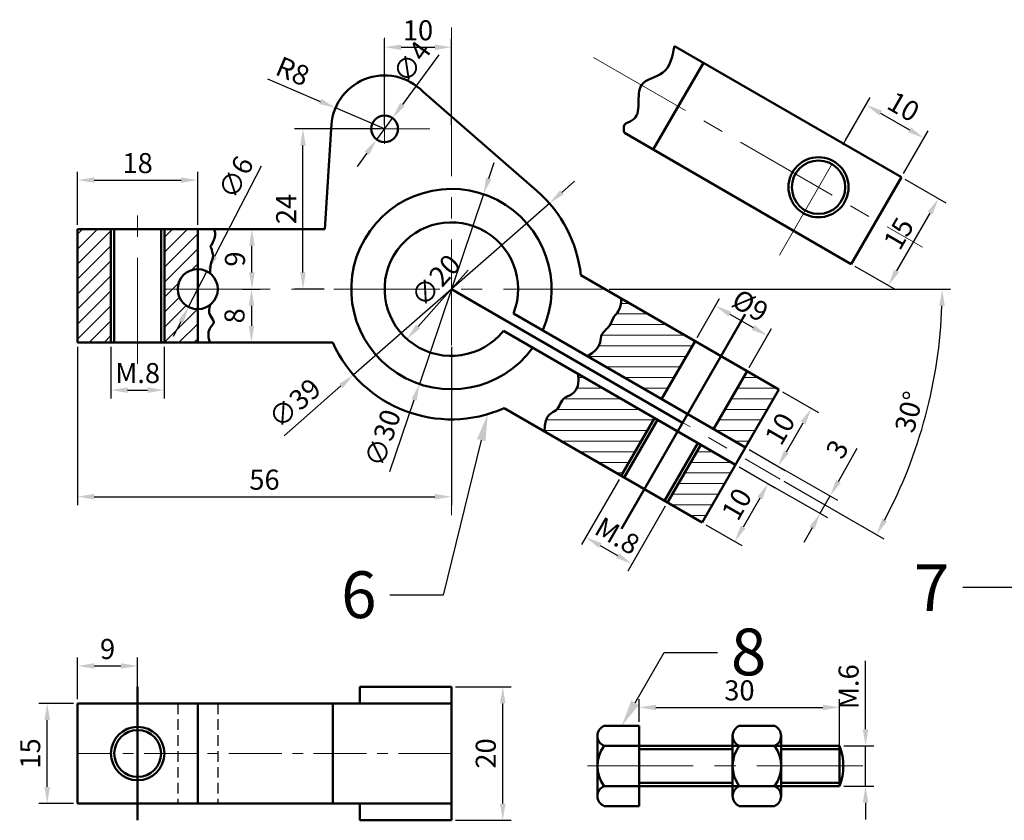
# Model space of a CAD drawing. Units: millimetres. Extents: x 77 to 718, y -35 to 313.
# Tile 5 of 7: x 386 to 533, y 99 to 219. Entities that reach past the tile are written whole.
import ezdxf
from ezdxf import colors
from ezdxf.entities.mleader import LeaderData, LeaderLine
from ezdxf.math import Vec2, Vec3

# ---------------------------------------------------------------- set-up
doc = ezdxf.new("R2010")
doc.units = ezdxf.units.MM
doc.header["$LTSCALE"] = 0.5
doc.linetypes.add('CENTER', pattern=[50.8, 31.75, -6.35, 6.35, -6.35])
doc.linetypes.add('HIDDEN', pattern=[9.525, 6.35, -3.175])
for name, color, linetype, lineweight in [('M-CNTR', 1, 'CENTER', 18), ('M-DIMS', 2, 'Continuous', 25), ('M-HATC', 8, 'Continuous', 18), ('M-HIDN', 8, 'HIDDEN', 25), ('M-OUTL', 7, 'Continuous', 50), ('M-TEXT', 3, 'Continuous', 25)]:
    doc.layers.add(name, color=color, linetype=linetype, lineweight=lineweight)
doc.styles.get("Standard").update_dxf_attribs({"font": 'arial.ttf'})
doc.dimstyles.new('ISO-25', dxfattribs={"dimtxt": 3, "dimasz": 2.5, "dimexe": 1.25, "dimexo": 0.625, "dimtad": 1, "dimtxsty": 'Standard', "dimcen": 2.5, "dimadec": 0, "dimazin": 0, "dimtfac": 1, "dimtmove": 0, "dimatfit": 3, "dimfxl": 1, "dimarcsym": 0})

# ---------------------------------------------------------------- blocks, each defined once
blk = doc.blocks.new('*D67')
at = {"layer": 'Defpoints', "color": 0, "transparency": 16777216}
for p in [(412.28, 195.29), (394.28, 187.97), (412.28, 187.97)]:
    blk.add_point(p, dxfattribs=at)
at = {"layer": 'M-DIMS', "color": 0, "lineweight": -2, "transparency": 16777216}
for p, q in [((394.28, 188.59), (394.28, 196.54)), ((412.28, 188.59), (412.28, 196.54)), ((396.78, 195.29), (409.78, 195.29))]:
    blk.add_line(p, q, dxfattribs=at)
at = {"layer": 'M-DIMS', "color": 0, "transparency": 16777216}
for points in [[(396.78, 195.71), (396.78, 194.88), (394.28, 195.29)], [(409.78, 195.71), (409.78, 194.88), (412.28, 195.29)]]:
    blk.add_solid(points, dxfattribs=at)
at = {"layer": 'M-DIMS', "color": 0, "transparency": 16777216, "insert": (403.28, 197.45), "char_height": 3, "attachment_point": 5}
blk.add_mtext('18', dxfattribs=at)
blk = doc.blocks.new('*D68')
at = {"layer": 'Defpoints', "color": 0, "transparency": 16777216}
for p in [(428.05, 202.97), (440.28, 202.97), (431.83, 178.97)]:
    blk.add_point(p, dxfattribs=at)
at = {"layer": 'M-DIMS', "color": 0, "lineweight": -2, "transparency": 16777216}
for p, q in [((439.66, 202.97), (426.8, 202.97)), ((428.05, 181.47), (428.05, 200.47)), ((431.21, 178.97), (426.8, 178.97))]:
    blk.add_line(p, q, dxfattribs=at)
at = {"layer": 'M-DIMS', "color": 0, "transparency": 16777216}
for points in [[(427.64, 200.47), (428.47, 200.47), (428.05, 202.97)], [(427.64, 181.47), (428.47, 181.47), (428.05, 178.97)]]:
    blk.add_solid(points, dxfattribs=at)
at = {"layer": 'M-DIMS', "color": 0, "transparency": 16777216, "insert": (425.92, 190.97), "char_height": 3, "attachment_point": 5, "rotation": 90}
blk.add_mtext('24', dxfattribs=at)
blk = doc.blocks.new('*D69')
at = {"layer": 'Defpoints', "color": 0, "transparency": 16777216}
for p in [(450.28, 215.19), (440.28, 202.97), (450.28, 202.97)]:
    blk.add_point(p, dxfattribs=at)
at = {"layer": 'M-DIMS', "color": 0, "lineweight": -2, "transparency": 16777216}
for p, q in [((440.28, 203.59), (440.28, 216.44)), ((450.28, 203.59), (450.28, 216.44)), ((442.78, 215.19), (447.78, 215.19))]:
    blk.add_line(p, q, dxfattribs=at)
at = {"layer": 'M-DIMS', "color": 0, "transparency": 16777216}
for points in [[(442.78, 215.6), (442.78, 214.77), (440.28, 215.19)], [(447.78, 215.6), (447.78, 214.77), (450.28, 215.19)]]:
    blk.add_solid(points, dxfattribs=at)
at = {"layer": 'M-DIMS', "color": 0, "transparency": 16777216, "insert": (445.28, 217.34), "char_height": 3, "attachment_point": 5}
blk.add_mtext('10', dxfattribs=at)
blk = doc.blocks.new('*D70')
at = {"layer": 'Defpoints', "color": 0, "transparency": 16777216}
for p in [(399.28, 170.97), (407.28, 170.97), (407.28, 163.85)]:
    blk.add_point(p, dxfattribs=at)
at = {"layer": 'M-DIMS', "color": 0, "lineweight": -2, "transparency": 16777216}
for p, q in [((399.28, 170.34), (399.28, 162.6)), ((407.28, 170.34), (407.28, 162.6)), ((401.78, 163.85), (404.78, 163.85))]:
    blk.add_line(p, q, dxfattribs=at)
at = {"layer": 'M-DIMS', "color": 0, "transparency": 16777216}
for points in [[(401.78, 164.27), (401.78, 163.43), (399.28, 163.85)], [(404.78, 164.27), (404.78, 163.43), (407.28, 163.85)]]:
    blk.add_solid(points, dxfattribs=at)
at = {"layer": 'M-DIMS', "color": 0, "transparency": 16777216, "insert": (403.28, 166.01), "char_height": 3, "attachment_point": 5}
blk.add_mtext('M.8', dxfattribs=at)
blk = doc.blocks.new('*D71')
at = {"layer": 'Defpoints', "color": 0, "transparency": 16777216}
for p in [(418.39, 187.97), (420.41, 187.97), (418.39, 178.97)]:
    blk.add_point(p, dxfattribs=at)
at = {"layer": 'M-DIMS', "color": 0, "lineweight": -2, "transparency": 16777216}
for p, q in [((419.01, 187.97), (421.66, 187.97)), ((420.41, 181.47), (420.41, 185.47)), ((419.01, 178.97), (421.66, 178.97))]:
    blk.add_line(p, q, dxfattribs=at)
at = {"layer": 'M-DIMS', "color": 0, "transparency": 16777216}
for points in [[(419.99, 185.47), (420.82, 185.47), (420.41, 187.97)], [(419.99, 181.47), (420.82, 181.47), (420.41, 178.97)]]:
    blk.add_solid(points, dxfattribs=at)
at = {"layer": 'M-DIMS', "color": 0, "transparency": 16777216, "insert": (418.25, 183.47), "char_height": 3, "attachment_point": 5, "rotation": 90}
blk.add_mtext('9', dxfattribs=at)
blk = doc.blocks.new('*D72')
at = {"layer": 'Defpoints', "color": 0, "transparency": 16777216}
for p in [(420.33, 178.97), (420.33, 170.97), (420.33, 170.97)]:
    blk.add_point(p, dxfattribs=at)
at = {"layer": 'M-DIMS', "color": 0, "lineweight": -2, "transparency": 16777216}
for p, q in [((420.96, 178.97), (421.58, 178.97)), ((420.33, 176.47), (420.33, 173.47)), ((420.96, 170.97), (421.58, 170.97))]:
    blk.add_line(p, q, dxfattribs=at)
at = {"layer": 'M-DIMS', "color": 0, "transparency": 16777216}
for points in [[(419.92, 176.47), (420.75, 176.47), (420.33, 178.97)], [(419.92, 173.47), (420.75, 173.47), (420.33, 170.97)]]:
    blk.add_solid(points, dxfattribs=at)
at = {"layer": 'M-DIMS', "color": 0, "transparency": 16777216, "insert": (418.18, 174.97), "char_height": 3, "attachment_point": 5, "rotation": 90}
blk.add_mtext('8', dxfattribs=at)
blk = doc.blocks.new('*D73')
at = {"layer": 'Defpoints', "color": 0, "transparency": 16777216}
for p in [(499.34, 163.93), (504.21, 161.11), (494.34, 155.27)]:
    blk.add_point(p, dxfattribs=at)
at = {"layer": 'M-DIMS', "color": 0, "lineweight": -2, "transparency": 16777216}
for p, q in [((499.88, 163.61), (505.29, 160.49)), ((500.46, 154.62), (502.96, 158.95)), ((494.88, 154.95), (500.29, 151.83))]:
    blk.add_line(p, q, dxfattribs=at)
at = {"layer": 'M-DIMS', "color": 0, "transparency": 16777216}
for points in [[(502.6, 159.16), (503.32, 158.74), (504.21, 161.11)], [(500.1, 154.83), (500.82, 154.41), (499.21, 152.45)]]:
    blk.add_solid(points, dxfattribs=at)
at = {"layer": 'M-DIMS', "color": 0, "transparency": 16777216, "insert": (499.84, 157.86), "char_height": 3, "attachment_point": 5, "rotation": 60}
blk.add_mtext('10', dxfattribs=at)
blk = doc.blocks.new('*D74')
at = {"layer": 'Defpoints', "color": 0, "transparency": 16777216}
for p in [(492.84, 152.67), (487.84, 144.01), (492.73, 141.18)]:
    blk.add_point(p, dxfattribs=at)
at = {"layer": 'M-DIMS', "color": 0, "lineweight": -2, "transparency": 16777216}
for p, q in [((493.38, 152.36), (498.81, 149.22)), ((496.48, 147.68), (493.98, 143.35)), ((488.38, 143.7), (493.81, 140.56))]:
    blk.add_line(p, q, dxfattribs=at)
at = {"layer": 'M-DIMS', "color": 0, "transparency": 16777216}
for points in [[(496.12, 147.89), (496.84, 147.47), (497.73, 149.84)], [(493.62, 143.56), (494.34, 143.14), (492.73, 141.18)]]:
    blk.add_solid(points, dxfattribs=at)
at = {"layer": 'M-DIMS', "color": 0, "transparency": 16777216, "insert": (493.36, 146.59), "char_height": 3, "attachment_point": 5, "rotation": 60}
blk.add_mtext('10', dxfattribs=at)
blk = doc.blocks.new('*D75')
at = {"layer": 'Defpoints', "color": 0, "transparency": 16777216}
for p in [(499.21, 152.45), (497.73, 149.84), (507.03, 148.01)]:
    blk.add_point(p, dxfattribs=at)
at = {"layer": 'M-DIMS', "color": 0, "lineweight": -2, "transparency": 16777216}
for p, q in [((508.26, 150.18), (511.09, 155.15)), ((499.75, 152.14), (508.11, 147.39)), ((498.27, 149.54), (506.63, 144.78)), ((505.54, 145.4), (507.03, 148.01)), ((504.31, 143.23), (503.07, 141.05))]:
    blk.add_line(p, q, dxfattribs=at)
at = {"layer": 'M-DIMS', "color": 0, "transparency": 16777216}
for points in [[(507.9, 150.39), (508.62, 149.97), (507.03, 148.01)], [(503.94, 143.43), (504.67, 143.02), (505.54, 145.4)]]:
    blk.add_solid(points, dxfattribs=at)
at = {"layer": 'M-DIMS', "color": 0, "transparency": 16777216, "insert": (508.42, 154.82), "char_height": 3, "attachment_point": 5, "rotation": 60.3651}
blk.add_mtext('3', dxfattribs=at)
blk = doc.blocks.new('*D76')
at = {"layer": 'Defpoints', "color": 0, "transparency": 16777216}
for p in [(486.78, 171.18), (497.63, 171.98), (494.57, 166.68)]:
    blk.add_point(p, dxfattribs=at)
at = {"layer": 'M-DIMS', "color": 0, "lineweight": -2, "transparency": 16777216}
for p, q in [((487.09, 171.72), (490.46, 177.56)), ((492, 175.23), (495.47, 173.23)), ((494.88, 167.22), (498.26, 173.06))]:
    blk.add_line(p, q, dxfattribs=at)
at = {"layer": 'M-DIMS', "color": 0, "transparency": 16777216}
for points in [[(492.21, 175.59), (491.8, 174.87), (489.84, 176.48)], [(495.68, 173.59), (495.26, 172.87), (497.63, 171.98)]]:
    blk.add_solid(points, dxfattribs=at)
at = {"layer": 'M-DIMS', "color": 0, "transparency": 16777216, "insert": (494.86, 176.17), "char_height": 3, "attachment_point": 5, "rotation": 330}
blk.add_mtext('%%C9', dxfattribs=at)
blk = doc.blocks.new('*D77')
at = {"layer": 'Defpoints', "color": 0, "transparency": 16777216}
for p in [(517.69, 195.72), (523.24, 192.51), (510.19, 182.73)]:
    blk.add_point(p, dxfattribs=at)
at = {"layer": 'M-DIMS', "color": 0, "lineweight": -2, "transparency": 16777216}
for p, q in [((518.23, 195.41), (524.33, 191.89)), ((516.99, 181.69), (521.99, 190.35)), ((510.73, 182.42), (516.83, 178.9))]:
    blk.add_line(p, q, dxfattribs=at)
at = {"layer": 'M-DIMS', "color": 0, "transparency": 16777216}
for points in [[(521.63, 190.56), (522.35, 190.14), (523.24, 192.51)], [(516.63, 181.9), (517.35, 181.48), (515.74, 179.52)]]:
    blk.add_solid(points, dxfattribs=at)
at = {"layer": 'M-DIMS', "color": 0, "transparency": 16777216, "insert": (517.62, 187.1), "char_height": 3, "attachment_point": 5, "rotation": 60}
blk.add_mtext('15', dxfattribs=at)
blk = doc.blocks.new('*D78')
at = {"layer": 'Defpoints', "color": 0, "transparency": 16777216}
for p in [(475.71, 151.01), (482.64, 147.01), (477.34, 137.83)]:
    blk.add_point(p, dxfattribs=at)
at = {"layer": 'M-DIMS', "color": 0, "lineweight": -2, "transparency": 16777216}
for p, q in [((475.4, 150.47), (469.79, 140.75)), ((482.33, 146.47), (476.71, 136.75)), ((472.58, 140.58), (475.17, 139.08))]:
    blk.add_line(p, q, dxfattribs=at)
at = {"layer": 'M-DIMS', "color": 0, "transparency": 16777216}
for points in [[(472.78, 140.94), (472.37, 140.22), (470.41, 141.83)], [(475.38, 139.44), (474.97, 138.72), (477.34, 137.83)]]:
    blk.add_solid(points, dxfattribs=at)
at = {"layer": 'M-DIMS', "color": 0, "transparency": 16777216, "insert": (474.95, 141.7), "char_height": 3, "attachment_point": 5, "rotation": 330}
blk.add_mtext('M.8', dxfattribs=at)
blk = doc.blocks.new('*D79')
at = {"layer": 'Defpoints', "color": 0, "transparency": 16777216}
for p in [(407.28, 178.97), (450.28, 178.97), (473.28, 178.97), (519.38, 153.82), (499.54, 150.53)]:
    blk.add_point(p, dxfattribs=at)
at = {"layer": 'M-DIMS', "color": 0, "lineweight": -2, "transparency": 16777216}
for p, q in [((473.91, 178.97), (525.07, 178.97)), ((500.08, 150.22), (515.05, 141.58))]:
    blk.add_line(p, q, dxfattribs=at)
blk.add_arc((450.28, 178.97), 73.53, 331.948, 358.052, dxfattribs=at)
at = {"layer": 'M-DIMS', "color": 0, "transparency": 16777216}
for points in [[(523.36, 176.48), (524.19, 176.46), (523.82, 178.97)], [(515.54, 144.18), (514.81, 144.59), (513.97, 142.2)]]:
    blk.add_solid(points, dxfattribs=at)
at = {"layer": 'M-DIMS', "color": 0, "transparency": 16777216, "insert": (519.23, 160.49), "char_height": 3, "attachment_point": 5, "rotation": 75}
blk.add_mtext('30°', dxfattribs=at)
blk = doc.blocks.new('*D80')
at = {"layer": 'Defpoints', "color": 0, "transparency": 16777216}
for p in [(509.03, 200.72), (521.07, 201.58), (517.69, 195.72)]:
    blk.add_point(p, dxfattribs=at)
at = {"layer": 'M-DIMS', "color": 0, "lineweight": -2, "transparency": 16777216}
for p, q in [((509.34, 201.26), (513.04, 207.66)), ((514.58, 205.33), (518.91, 202.83)), ((518, 196.26), (521.7, 202.66))]:
    blk.add_line(p, q, dxfattribs=at)
at = {"layer": 'M-DIMS', "color": 0, "transparency": 16777216}
for points in [[(514.79, 205.69), (514.37, 204.97), (512.41, 206.58)], [(519.12, 203.19), (518.7, 202.47), (521.07, 201.58)]]:
    blk.add_solid(points, dxfattribs=at)
at = {"layer": 'M-DIMS', "color": 0, "transparency": 16777216, "insert": (517.82, 205.95), "char_height": 3, "attachment_point": 5, "rotation": 330}
blk.add_mtext('10', dxfattribs=at)
blk = doc.blocks.new('*D81')
at = {"layer": 'Defpoints', "color": 0, "transparency": 16777216}
for p in [(394.28, 170.97), (450.28, 170.97), (450.28, 147.89)]:
    blk.add_point(p, dxfattribs=at)
at = {"layer": 'M-DIMS', "color": 0, "lineweight": -2, "transparency": 16777216}
for p, q in [((394.28, 170.34), (394.28, 146.64)), ((450.28, 170.34), (450.28, 146.64)), ((396.78, 147.89), (447.78, 147.89))]:
    blk.add_line(p, q, dxfattribs=at)
at = {"layer": 'M-DIMS', "color": 0, "transparency": 16777216}
for points in [[(396.78, 148.31), (396.78, 147.47), (394.28, 147.89)], [(447.78, 148.31), (447.78, 147.47), (450.28, 147.89)]]:
    blk.add_solid(points, dxfattribs=at)
at = {"layer": 'M-DIMS', "color": 0, "transparency": 16777216, "insert": (422.28, 150.05), "char_height": 3, "attachment_point": 5}
blk.add_mtext('56', dxfattribs=at)
blk = doc.blocks.new('*D82')
at = {"layer": 'Defpoints', "color": 0, "transparency": 16777216}
for p in [(456.94, 186.43), (443.63, 171.51)]:
    blk.add_point(p, dxfattribs=at)
at = {"layer": 'M-DIMS', "color": 0, "lineweight": -2, "transparency": 16777216}
blk.add_line((452.81, 181.8), (445.29, 173.37), dxfattribs=at)
at = {"layer": 'M-DIMS', "color": 0, "transparency": 16777216}
blk.add_solid([(444.98, 173.65), (445.6, 173.09), (443.63, 171.51)], dxfattribs=at)
at = {"layer": 'M-DIMS', "color": 0, "transparency": 16777216, "insert": (448.21, 180.01), "char_height": 3, "attachment_point": 5, "rotation": 48.266}
blk.add_mtext('∅20', dxfattribs=at)
blk = doc.blocks.new('*D83')
at = {"layer": 'Defpoints', "color": 0, "transparency": 16777216}
for p in [(455.08, 193.18), (445.49, 164.75)]:
    blk.add_point(p, dxfattribs=at)
at = {"layer": 'M-DIMS', "color": 0, "lineweight": -2, "transparency": 16777216}
for p, q in [((455.88, 195.55), (456.68, 197.92)), ((455.08, 193.18), (445.49, 164.75)), ((441.08, 151.68), (444.69, 162.39))]:
    blk.add_line(p, q, dxfattribs=at)
at = {"layer": 'M-DIMS', "color": 0, "transparency": 16777216}
for points in [[(455.48, 195.68), (456.27, 195.42), (455.08, 193.18)], [(444.3, 162.52), (445.09, 162.25), (445.49, 164.75)]]:
    blk.add_solid(points, dxfattribs=at)
at = {"layer": 'M-DIMS', "color": 0, "transparency": 16777216, "insert": (440.36, 156.56), "char_height": 3, "attachment_point": 5, "rotation": 71.3582}
blk.add_mtext('∅30', dxfattribs=at)
blk = doc.blocks.new('*D84')
at = {"layer": 'Defpoints', "color": 0, "transparency": 16777216}
for p in [(464.96, 191.81), (435.61, 166.12)]:
    blk.add_point(p, dxfattribs=at)
at = {"layer": 'M-DIMS', "color": 0, "lineweight": -2, "transparency": 16777216}
for p, q in [((466.84, 193.46), (468.72, 195.11)), ((464.96, 191.81), (435.61, 166.12)), ((425.22, 157.02), (433.73, 164.48))]:
    blk.add_line(p, q, dxfattribs=at)
at = {"layer": 'M-DIMS', "color": 0, "transparency": 16777216}
for points in [[(466.56, 193.77), (467.11, 193.15), (464.96, 191.81)], [(433.46, 164.79), (434.01, 164.16), (435.61, 166.12)]]:
    blk.add_solid(points, dxfattribs=at)
at = {"layer": 'M-DIMS', "color": 0, "transparency": 16777216, "insert": (427.06, 161.61), "char_height": 3, "attachment_point": 5, "rotation": 41.2003}
blk.add_mtext('∅39', dxfattribs=at)
blk = doc.blocks.new('*D85')
at = {"layer": 'Defpoints', "color": 0, "transparency": 16777216}
for p in [(441.46, 204.58), (439.1, 201.35)]:
    blk.add_point(p, dxfattribs=at)
at = {"layer": 'M-DIMS', "color": 0, "lineweight": -2, "transparency": 16777216}
for p, q in [((448.38, 214.05), (442.94, 206.6)), ((439.1, 201.35), (441.46, 204.58)), ((437.63, 199.33), (436.16, 197.32))]:
    blk.add_line(p, q, dxfattribs=at)
at = {"layer": 'M-DIMS', "color": 0, "transparency": 16777216}
for points in [[(442.6, 206.85), (443.28, 206.36), (441.46, 204.58)], [(437.29, 199.58), (437.97, 199.09), (439.1, 201.35)]]:
    blk.add_solid(points, dxfattribs=at)
at = {"layer": 'M-DIMS', "color": 0, "transparency": 16777216, "insert": (444.66, 212.76), "char_height": 3, "attachment_point": 5, "rotation": 53.8527}
blk.add_mtext('∅4', dxfattribs=at)
blk = doc.blocks.new('*D86')
at = {"layer": 'Defpoints', "color": 0, "transparency": 16777216}
for p in [(432.92, 206.1), (440.28, 202.97)]:
    blk.add_point(p, dxfattribs=at)
at = {"layer": 'M-DIMS', "color": 0, "lineweight": -2, "transparency": 16777216}
for p, q in [((422.72, 210.45), (430.62, 207.08)), ((440.28, 202.97), (432.92, 206.1))]:
    blk.add_line(p, q, dxfattribs=at)
at = {"layer": 'M-DIMS', "color": 0, "transparency": 16777216}
blk.add_solid([(430.79, 207.47), (430.46, 206.7), (432.92, 206.1)], dxfattribs=at)
at = {"layer": 'M-DIMS', "color": 0, "transparency": 16777216, "insert": (426.37, 211.24), "char_height": 3, "attachment_point": 5, "rotation": 336.9265}
blk.add_mtext('R8', dxfattribs=at)
blk = doc.blocks.new('*D87')
at = {"layer": 'Defpoints', "color": 0, "transparency": 16777216}
for p in [(413.66, 181.63), (410.91, 176.3)]:
    blk.add_point(p, dxfattribs=at)
at = {"layer": 'M-DIMS', "color": 0, "lineweight": -2, "transparency": 16777216}
for p, q in [((421.81, 197.38), (414.81, 183.85)), ((410.91, 176.3), (413.66, 181.63)), ((409.76, 174.08), (408.61, 171.86))]:
    blk.add_line(p, q, dxfattribs=at)
at = {"layer": 'M-DIMS', "color": 0, "transparency": 16777216}
for points in [[(414.44, 184.04), (415.18, 183.66), (413.66, 181.63)], [(409.39, 174.27), (410.13, 173.89), (410.91, 176.3)]]:
    blk.add_solid(points, dxfattribs=at)
at = {"layer": 'M-DIMS', "color": 0, "transparency": 16777216, "insert": (418.34, 195.53), "char_height": 3, "attachment_point": 5, "rotation": 62.6333}
blk.add_mtext('∅6', dxfattribs=at)
blk = doc.blocks.new('*D101')
at = {"layer": 'Defpoints', "color": 0, "ltscale": 0.5, "transparency": 16777216}
for p in [(450.28, 119.44), (457.98, 119.44), (450.28, 99.44)]:
    blk.add_point(p, dxfattribs=at)
at = {"layer": 'M-DIMS', "color": 0, "lineweight": -2, "ltscale": 0.5, "transparency": 16777216}
for p, q in [((450.91, 119.44), (459.23, 119.44)), ((457.98, 101.94), (457.98, 116.94)), ((450.91, 99.44), (459.23, 99.44))]:
    blk.add_line(p, q, dxfattribs=at)
at = {"layer": 'M-DIMS', "color": 0, "ltscale": 0.5, "transparency": 16777216}
for points in [[(457.56, 116.94), (458.4, 116.94), (457.98, 119.44)], [(457.56, 101.94), (458.4, 101.94), (457.98, 99.44)]]:
    blk.add_solid(points, dxfattribs=at)
at = {"layer": 'M-DIMS', "color": 0, "ltscale": 0.5, "transparency": 16777216, "insert": (455.82, 109.44), "char_height": 3, "attachment_point": 5, "rotation": 90}
blk.add_mtext('20', dxfattribs=at)
blk = doc.blocks.new('*D102')
at = {"layer": 'Defpoints', "color": 0, "ltscale": 0.5, "transparency": 16777216}
for p in [(403.28, 122.54), (394.28, 116.94), (403.28, 116.94)]:
    blk.add_point(p, dxfattribs=at)
at = {"layer": 'M-DIMS', "color": 0, "lineweight": -2, "ltscale": 0.5, "transparency": 16777216}
for p, q in [((394.28, 117.56), (394.28, 123.79)), ((396.78, 122.54), (400.78, 122.54)), ((403.28, 117.56), (403.28, 123.79))]:
    blk.add_line(p, q, dxfattribs=at)
at = {"layer": 'M-DIMS', "color": 0, "ltscale": 0.5, "transparency": 16777216}
for points in [[(396.78, 122.96), (396.78, 122.13), (394.28, 122.54)], [(400.78, 122.96), (400.78, 122.13), (403.28, 122.54)]]:
    blk.add_solid(points, dxfattribs=at)
at = {"layer": 'M-DIMS', "color": 0, "ltscale": 0.5, "transparency": 16777216, "insert": (398.78, 124.7), "char_height": 3, "attachment_point": 5}
blk.add_mtext('9', dxfattribs=at)
blk = doc.blocks.new('*D103')
at = {"layer": 'Defpoints', "color": 0, "ltscale": 0.5, "transparency": 16777216}
for p in [(389.74, 116.94), (394.28, 116.94), (394.28, 101.94)]:
    blk.add_point(p, dxfattribs=at)
at = {"layer": 'M-DIMS', "color": 0, "lineweight": -2, "ltscale": 0.5, "transparency": 16777216}
for p, q in [((393.66, 116.94), (388.49, 116.94)), ((389.74, 104.44), (389.74, 114.44)), ((393.66, 101.94), (388.49, 101.94))]:
    blk.add_line(p, q, dxfattribs=at)
at = {"layer": 'M-DIMS', "color": 0, "ltscale": 0.5, "transparency": 16777216}
for points in [[(389.32, 114.44), (390.16, 114.44), (389.74, 116.94)], [(389.32, 104.44), (390.16, 104.44), (389.74, 101.94)]]:
    blk.add_solid(points, dxfattribs=at)
at = {"layer": 'M-DIMS', "color": 0, "ltscale": 0.5, "transparency": 16777216, "insert": (387.58, 109.44), "char_height": 3, "attachment_point": 5, "rotation": 90}
blk.add_mtext('15', dxfattribs=at)
blk = doc.blocks.new('*U118')
at = {"layer": 'M-CNTR', "color": 0, "transparency": 16777216}
blk.add_line((16.63, 0), (-26.03, 0), dxfattribs=at)
blk = doc.blocks.new('*D125')
at = {"layer": 'Defpoints', "color": 0, "ltscale": 0.5, "transparency": 16777216}
for p in [(508.43, 110.57), (508.43, 104.57), (512.32, 104.57)]:
    blk.add_point(p, dxfattribs=at)
at = {"layer": 'M-DIMS', "color": 0, "lineweight": -2, "ltscale": 0.5, "transparency": 16777216}
for p, q in [((512.32, 113.07), (512.32, 123.3)), ((509.05, 110.57), (513.57, 110.57)), ((512.32, 104.57), (512.32, 110.57)), ((509.05, 104.57), (513.57, 104.57)), ((512.32, 102.07), (512.32, 99.57))]:
    blk.add_line(p, q, dxfattribs=at)
at = {"layer": 'M-DIMS', "color": 0, "ltscale": 0.5, "transparency": 16777216}
for points in [[(511.91, 113.07), (512.74, 113.07), (512.32, 110.57)], [(511.91, 102.07), (512.74, 102.07), (512.32, 104.57)]]:
    blk.add_solid(points, dxfattribs=at)
at = {"layer": 'M-DIMS', "color": 0, "ltscale": 0.5, "transparency": 16777216, "insert": (510.17, 119.43), "char_height": 3, "attachment_point": 5, "rotation": 90}
blk.add_mtext('M.6', dxfattribs=at)
blk = doc.blocks.new('*D126')
at = {"layer": 'Defpoints', "color": 0, "ltscale": 0.5, "transparency": 16777216}
for p in [(508.43, 116.34), (478.43, 113.57), (508.43, 107.57)]:
    blk.add_point(p, dxfattribs=at)
at = {"layer": 'M-DIMS', "color": 0, "lineweight": -2, "ltscale": 0.5, "transparency": 16777216}
for p, q in [((478.43, 114.19), (478.43, 117.59)), ((508.43, 108.19), (508.43, 117.59)), ((480.93, 116.34), (505.93, 116.34))]:
    blk.add_line(p, q, dxfattribs=at)
at = {"layer": 'M-DIMS', "color": 0, "ltscale": 0.5, "transparency": 16777216}
for points in [[(480.93, 116.75), (480.93, 115.92), (478.43, 116.34)], [(505.93, 116.75), (505.93, 115.92), (508.43, 116.34)]]:
    blk.add_solid(points, dxfattribs=at)
at = {"layer": 'M-DIMS', "color": 0, "ltscale": 0.5, "transparency": 16777216, "insert": (493.43, 118.5), "char_height": 3, "attachment_point": 5}
blk.add_mtext('30', dxfattribs=at)
blk = doc.blocks.new('SHUNT-TERMINAL')
for p, q in [((19.31, 22.65), (54.05, 2.6)), ((17.81, 20.06), (52.55, 0))]:
    blk.add_line(p, q)
blk.add_arc((10, 26.3), 10, 338.6269, 321.3731)

msp = doc.modelspace()

# ---------------------------------------------------------------- hatches: boundary and pattern name
at = {"layer": 'M-HATC'}
h = msp.add_hatch(dxfattribs=at)
h.set_pattern_fill('ANSI31', color=256, scale=0.5)
h.set_pattern_definition([(45, (-118.3937, 56.1893), (-1.122532, 1.122532), [])])
h.paths.add_polyline_path([(399.284, 187.968), (394.284, 187.968), (394.284, 170.968), (399.284, 170.968)])
h.paths.add_polyline_path([(412.284, 187.968), (407.284, 187.968), (407.284, 178.968), (409.284, 178.968, -0.4142136), (412.284, 181.968)])
h.paths.add_polyline_path([(409.284, 178.968), (407.284, 178.968), (407.284, 170.968), (412.284, 170.968), (412.284, 175.968, -0.4142136)])
h = msp.add_hatch(dxfattribs=at)
h.set_pattern_fill('ANSI31', color=256, scale=0.5, angle=135)
h.set_pattern_definition([(180, (-118.3937, 56.1893), (-1e-16, -1.5875), [])])
edge = h.paths.add_edge_path()
edge.add_line((470.683, 168.923), (481.778, 162.517))
edge.add_line((481.778, 162.517), (486.778, 171.177))
edge.add_line((486.778, 171.177), (475.729, 177.556))
edge.add_spline(control_points=[(475.729, 177.556), (475.729, 175.754), (474.299, 174.928), (474.299, 173.406), (472.272, 172.236), (472.807, 170.149), (470.683, 168.923)], knot_values=[0, 0, 0, 0, 1, 2, 3, 4, 4, 4, 4], degree=3, periodic=0)
edge = h.paths.add_edge_path()
edge.add_line((480.711, 159.669), (469.297, 166.259))
edge.add_spline(control_points=[(469.297, 166.259), (469.579, 163.217), (466.562, 163.217), (466.562, 160.377), (464.229, 160.377), (464.229, 157.637)], knot_values=[0, 0, 0, 0, 1, 2, 3, 3, 3, 3], degree=3, periodic=0)
edge.add_line((464.229, 157.637), (475.711, 151.008))
edge.add_line((475.711, 151.008), (480.711, 159.669))
h.paths.add_polyline_path([(489.572, 158.017), (494.335, 155.267), (499.335, 163.927), (494.572, 166.677)])
h.paths.add_polyline_path([(482.639, 147.008), (487.835, 144.008), (492.835, 152.669), (487.639, 155.669)])

# ---------------------------------------------------------------- linework, layer by layer
at = {"layer": 'M-CNTR'}
for p, q in [((450.284, 145.106), (450.284, 218.776)), ((440.284, 216.61), (440.284, 197.905)), ((471.59, 213.674), (520.838, 185.24)), ((499.418, 184.07), (511.671, 205.293)), ((433.514, 202.968), (447.055, 202.968)), ((403.284, 167.769), (403.284, 190.711)), ((407.284, 178.968), (473.284, 178.968)), ((450.284, 178.968), (499.543, 150.528))]:
    msp.add_line(p, q, dxfattribs=at)
at = {"layer": 'M-CNTR', "ltscale": 0.5}
msp.add_line((450.284, 109.435), (394.284, 109.435), dxfattribs=at)
at = {"layer": 'M-HIDN', "ltscale": 0.5}
for p, q in [((409.284, 116.935), (409.284, 101.935)), ((415.284, 116.935), (415.284, 101.935))]:
    msp.add_line(p, q, dxfattribs=at)
at = {"layer": 'M-OUTL'}
for p, q in [((483.697, 215.344), (517.69, 195.718)), ((480.527, 199.854), (488.027, 212.844)), ((446.034, 208.531), (463.092, 193.672)), ((432.284, 202.968), (431.347, 187.968)), ((476.197, 202.354), (510.19, 182.728)), ((510.19, 182.728), (517.69, 195.718)), ((394.284, 187.968), (431.347, 187.968)), ((394.284, 170.968), (394.284, 187.968)), ((399.284, 170.968), (399.284, 187.968)), ((399.784, 170.968), (399.784, 187.968)), ((406.784, 170.968), (406.784, 187.968)), ((407.284, 170.968), (407.284, 187.968)), ((412.284, 170.968), (412.284, 187.968)), ((469.672, 181.053), (499.335, 163.927)), ((450.284, 178.968), (484.925, 158.968)), ((475.764, 143.101), (494.299, 175.204)), ((481.778, 162.517), (486.778, 171.177)), ((394.284, 170.968), (432.501, 170.968)), ((489.572, 158.017), (494.572, 166.677)), ((487.835, 144.008), (499.335, 163.927)), ((458.172, 161.134), (487.835, 144.008)), ((475.711, 151.008), (480.711, 159.669)), ((476.144, 150.758), (481.144, 159.419)), ((482.206, 147.258), (487.206, 155.919)), ((482.639, 147.008), (487.639, 155.669))]:
    msp.add_line(p, q, dxfattribs=at)
at = {"layer": 'M-OUTL', "ltscale": 0.5}
for p, q in [((403.284, 99.435), (403.284, 119.435)), ((436.569, 119.435), (450.284, 119.435)), ((436.569, 116.935), (436.569, 119.435)), ((450.284, 119.435), (450.284, 99.435)), ((394.284, 101.935), (394.284, 116.935)), ((394.284, 116.935), (450.284, 116.935)), ((412.284, 116.935), (412.284, 101.935)), ((432.525, 116.935), (432.525, 101.935)), ((478.425, 113.568), (473.164, 113.568)), ((478.425, 113.568), (478.425, 101.568)), ((498.677, 113.568), (493.416, 113.568)), ((472.164, 112.068), (472.164, 103.068)), ((492.416, 112.068), (492.416, 103.068)), ((499.677, 112.068), (499.677, 103.068)), ((482.164, 110.568), (473.164, 110.568)), ((478.425, 110.068), (492.416, 110.068)), ((482.164, 110.568), (508.425, 110.568)), ((499.677, 110.068), (508.425, 110.068)), ((508.425, 110.568), (508.425, 104.568)), ((492.416, 105.068), (478.425, 105.068)), ((508.425, 105.068), (499.677, 105.068)), ((482.164, 104.568), (473.164, 104.568)), ((508.425, 104.568), (482.164, 104.568)), ((394.284, 101.935), (450.284, 101.935)), ((436.569, 99.435), (436.569, 101.935)), ((473.164, 101.568), (478.425, 101.568)), ((493.416, 101.568), (498.677, 101.568)), ((450.284, 99.435), (436.569, 99.435))]:
    msp.add_line(p, q, dxfattribs=at)
at = {"layer": 'M-OUTL'}
for centre, radius in [((440.284, 202.968), 2), ((505.28, 194.223), 4.5), ((505.28, 194.223), 4), ((412.284, 178.968), 3)]:
    msp.add_circle(centre, radius, dxfattribs=at)
at = {"layer": 'M-OUTL', "ltscale": 0.5}
for radius in [4, 3.5]:
    msp.add_circle((403.284, 109.435), radius, dxfattribs=at)
at = {"layer": 'M-OUTL'}
for centre, radius, start, end in [((440.284, 202.968), 8, 44.05473, 180), ((450.284, 178.968), 15, 335.73917, 324.26083), ((450.284, 178.968), 19.5, 6.13881, 48.94259), ((450.284, 178.968), 19.5, 204.22094, 293.86119)]:
    msp.add_arc(centre, radius, start, end, dxfattribs=at)
at = {"layer": 'M-OUTL', "ltscale": 0.5}
for centre, radius, start, end in [((473.789, 112.068), 1.625, 112.61986, 247.38014), ((494.041, 112.068), 1.625, 112.61986, 247.38014), ((498.052, 112.068), 1.625, 292.61986, 67.38014), ((477.164, 107.568), 5, 143.1301, 216.8699), ((497.416, 107.568), 5, 143.1301, 216.8699), ((494.677, 107.568), 5, 323.1301, 36.8699), ((500.7, 107.568), 8.288, 338.77795, 21.22205), ((473.789, 103.068), 1.625, 112.61986, 247.38014), ((494.041, 103.068), 1.625, 112.61986, 247.38014), ((498.052, 103.068), 1.625, 292.61986, 67.38014)]:
    msp.add_arc(centre, radius, start, end, dxfattribs=at)
at = {"layer": 'M-OUTL'}
for points, knots in [([(476.197, 202.354), (476.103, 202.812), (475.903, 203.792), (479.273, 204.463), (477.053, 210.134), (482.815, 210.89), (483.385, 213.77), (483.697, 215.344)], [0, 0, 0, 0, 1.2079265, 2.5818455, 8.041722, 11.6731455, 16.0513845, 16.0513845, 16.0513845, 16.0513845]), ([(414.642, 187.968), (414.852, 187.666), (415.117, 187.283), (414.179, 185.099), (414.139, 185.696), (414.748, 183.722), (414.166, 182.94), (414.156, 181.947), (414.15, 181.317)], [0, 0, 0, 0, 1.4548941, 1.8422114, 3.2453238, 4.2389274, 5.2482843, 7.0044557, 7.0044557, 7.0044557, 7.0044557]), ([(414.125, 176.599), (414.004, 176.067), (413.786, 175.137), (415.05, 174.079), (413.618, 172.845), (413.914, 171.708), (414.107, 170.968)], [11.7229323, 11.7229323, 11.7229323, 11.7229323, 13.2748884, 14.383373, 15.5275287, 17.6555518, 17.6555518, 17.6555518, 17.6555518])]:
    msp.add_open_spline(points, degree=3, knots=knots, dxfattribs=at)
for points in [[(470.683, 168.923), (472.807, 170.149), (472.272, 172.236), (474.299, 173.406), (474.299, 174.928), (475.729, 175.754), (475.729, 177.556)], [(464.229, 157.637), (464.229, 160.377), (466.562, 160.377), (466.562, 163.217), (469.579, 163.217), (469.297, 166.259)]]:
    msp.add_open_spline(points, degree=3, dxfattribs=at)

# ---------------------------------------------------------------- block references
at = {"layer": 'M-CNTR'}
msp.add_blockref('*U118', (495.295, 107.568), dxfattribs=at)
at = {"layer": 'M-OUTL'}
msp.add_blockref('SHUNT-TERMINAL', (440.283, 152.669), dxfattribs=at)

# ---------------------------------------------------------------- dimensions: what is measured, and where the dimension line sits
at = {"layer": 'M-DIMS'}
for base, p1, p2, picture, middle in [((450.284, 215.185), (440.284, 202.968), (450.284, 202.968), '*D69', (445.284, 217.342)), ((412.284, 195.292), (394.284, 187.968), (412.284, 187.968), '*D67', (403.284, 197.449)), ((450.284, 147.889), (394.284, 170.968), (450.284, 170.968), '*D81', (422.284, 150.046))]:
    dim = msp.add_linear_dim(base=base, p1=p1, p2=p2, dimstyle='ISO-25', override={"dimclrd": 0, "dimclre": 0, "dimclrt": 0}, dxfattribs=at)
    dim.commit()
    dim.dimension.update_dxf_attribs({"geometry": picture, "text_midpoint": middle})
for p1, p2, picture, middle in [((439.104, 201.353), (441.464, 204.583), '*D85', (446.47, 211.435)), ((410.905, 176.304), (413.663, 181.632), '*D87', (420.325, 194.503)), ((456.941, 186.43), (443.627, 171.505), '*D82', (449.885, 178.52))]:
    dim = msp.add_diameter_dim_2p(p1=p1, p2=p2, dimstyle='ISO-25', override={"dimclrd": 0, "dimclre": 0, "dimclrt": 0}, dxfattribs=at)
    dim.commit()
    dim.dimension.update_dxf_attribs({"geometry": picture, "text_midpoint": middle, "dimtype": 163})
dim = msp.add_radius_dim(center=(440.284, 202.968), mpoint=(432.924, 206.103), dimstyle='ISO-25', override={"dimclrd": 0, "dimclre": 0, "dimclrt": 0}, dxfattribs=at)
dim.commit()
dim.dimension.update_dxf_attribs({"geometry": '*D86', "text_midpoint": (426.366, 211.241)})
for p1, p2, distance, picture, middle in [((509.03, 200.718), (517.69, 195.718), 6.766, '*D80', (517.821, 205.945)), ((510.19, 182.728), (517.69, 195.718), -6.412, '*D77', (517.625, 187.096)), ((494.335, 155.267), (499.335, 163.927), -5.63, '*D73', (499.843, 157.86)), ((497.728, 149.844), (499.211, 152.452), -8.99, '*D75', (508.417, 154.816)), ((492.835, 152.669), (487.835, 144.008), 5.649, '*D74', (493.36, 146.592))]:
    dim = msp.add_aligned_dim(p1=p1, p2=p2, distance=distance, dimstyle='ISO-25', override={"dimclrd": 0, "dimclre": 0, "dimclrt": 0}, dxfattribs=at)
    dim.commit()
    dim.dimension.update_dxf_attribs({"geometry": picture, "text_midpoint": middle})
for base, p1, p2, picture, middle in [((428.054, 202.968), (431.832, 178.968), (440.284, 202.968), '*D68', (425.923, 190.968)), ((420.407, 187.968), (418.387, 178.968), (418.387, 187.968), '*D71', (418.25, 183.468)), ((420.334, 170.968), (420.334, 178.968), (420.334, 170.968), '*D72', (418.178, 174.968))]:
    dim = msp.add_linear_dim(base=base, p1=p1, p2=p2, angle=90, dimstyle='ISO-25', override={"dimclrd": 0, "dimclre": 0, "dimclrt": 0}, dxfattribs=at)
    dim.commit()
    dim.dimension.update_dxf_attribs({"geometry": picture, "text_midpoint": middle})
for p1, p2, picture, middle in [((455.079, 193.181), (445.489, 164.755), '*D83', (440.361, 156.564)), ((464.956, 191.812), (435.612, 166.123), '*D84', (427.057, 161.612))]:
    dim = msp.add_diameter_dim_2p(p1=p1, p2=p2, dimstyle='ISO-25', override={"dimclrd": 0, "dimclre": 0, "dimclrt": 0}, dxfattribs=at)
    dim.commit()
    dim.dimension.update_dxf_attribs({"geometry": picture, "text_midpoint": middle})
dim = msp.add_angular_dim_2l(base=(519.383, 153.818), line1=((450.284, 178.968), (499.543, 150.528)), line2=((407.284, 178.968), (473.284, 178.968)), dimstyle='ISO-25', override={"dimclrd": 0, "dimclre": 0, "dimclrt": 0}, dxfattribs=at)
dim.commit()
dim.dimension.update_dxf_attribs({"geometry": '*D79', "text_midpoint": (519.228, 160.494)})
for base, p1, p2, text, picture, middle in [((497.634, 171.98), (486.778, 171.177), (494.572, 166.677), '%%C<>', '*D76', (493.737, 174.23)), ((477.339, 137.829), (475.711, 151.008), (482.639, 147.008), 'M.<>', '*D78', (473.875, 139.829))]:
    dim = msp.add_linear_dim(base=base, p1=p1, p2=p2, angle=330, text=text, dimstyle='ISO-25', override={"dimclrd": 0, "dimclre": 0, "dimclrt": 0}, dxfattribs=at)
    dim.commit()
    dim.dimension.update_dxf_attribs({"geometry": picture, "text_midpoint": middle, "dimtype": 161})
dim = msp.add_linear_dim(base=(407.284, 163.851), p1=(399.284, 170.968), p2=(407.284, 170.968), text='M.<>', dimstyle='ISO-25', override={"dimclrd": 0, "dimclre": 0, "dimclrt": 0}, dxfattribs=at)
dim.commit()
dim.dimension.update_dxf_attribs({"geometry": '*D70', "text_midpoint": (403.284, 166.008)})
at = {"layer": 'M-DIMS', "ltscale": 0.5}
dim = msp.add_linear_dim(base=(403.284, 122.543), p1=(394.284, 116.935), p2=(403.284, 116.935), dimstyle='ISO-25', override={"dimclrd": 0, "dimclre": 0, "dimclrt": 0}, dxfattribs=at)
dim.commit()
dim.dimension.update_dxf_attribs({"geometry": '*D102', "text_midpoint": (398.784, 122.543), "dimtype": 160})
dim = msp.add_linear_dim(base=(512.322, 104.568), p1=(508.425, 110.568), p2=(508.425, 104.568), angle=90, text='M.<>', dimstyle='ISO-25', override={"dimclrd": 0, "dimclre": 0, "dimclrt": 0}, dxfattribs=at)
dim.commit()
dim.dimension.update_dxf_attribs({"geometry": '*D125', "text_midpoint": (512.322, 119.435), "dimtype": 160})
dim = msp.add_linear_dim(base=(508.425, 116.337), p1=(478.425, 113.568), p2=(508.425, 107.568), dimstyle='ISO-25', override={"dimclrd": 0, "dimclre": 0, "dimclrt": 0}, dxfattribs=at)
dim.commit()
dim.dimension.update_dxf_attribs({"geometry": '*D126', "text_midpoint": (493.425, 118.495)})
for base, p1, p2, picture, middle in [((457.979, 119.435), (450.284, 99.435), (450.284, 119.435), '*D101', (455.822, 109.435)), ((389.74, 116.935), (394.284, 101.935), (394.284, 116.935), '*D103', (387.583, 109.435))]:
    dim = msp.add_linear_dim(base=base, p1=p1, p2=p2, angle=90, dimstyle='ISO-25', override={"dimclrd": 0, "dimclre": 0, "dimclrt": 0}, dxfattribs=at)
    dim.commit()
    dim.dimension.update_dxf_attribs({"geometry": picture, "text_midpoint": middle})

# ---------------------------------------------------------------- leaders
at = {"layer": 'M-TEXT', "ltscale": 0.5}
ml = msp.add_multileader_mtext('Standard', dxfattribs=at)
ml.set_content('6', color=256)
ml.set_leader_properties()
ml.build(insert=Vec2(0, 0))
ctx = ml.context
ctx.base_point, ctx.char_height, ctx.plane_origin = Vec3(432.448, 133.158), 7, Vec3(455.719, 160.24)
ctx.text_align_type = 2
notes = []
notes.append((ctx, [(0, (1, 1, 0), (449.07, 133.158), (-1, 0), 8, [(0, [(455.719, 160.24)], 0, [])])]))
ctx.mtext.insert, ctx.mtext.alignment, ctx.mtext.flow_direction = Vec3(439.07, 136.717), 3, 5
ml = msp.add_multileader_mtext('Standard', dxfattribs=at)
ml.set_content('7', color=256)
ml.set_leader_properties()
ml.build(insert=Vec2(0, 0))
ctx = ml.context
ctx.base_point, ctx.char_height, ctx.plane_origin = Vec3(518.358, 134.277), 7, Vec3(547.915, 122.279)
ctx.text_align_type = 2
notes.append((ctx, [(0, (1, 1, 0), (534.889, 134.277), (-1, 0), 8, [(0, [(547.915, 122.279)], 0, [])])]))
ctx.mtext.insert, ctx.mtext.alignment, ctx.mtext.flow_direction = Vec3(524.889, 137.777), 3, 5
ml = msp.add_multileader_mtext('Standard', dxfattribs=at)
ml.set_content('8', color=256)
ml.set_leader_properties()
ml.build(insert=Vec2(0, 0))
ctx = ml.context
ctx.base_point, ctx.char_height, ctx.plane_origin = Vec3(490.153, 124.582), 7, Vec3(475.795, 113.568)
notes.append((ctx, [(0, (1, 1, 0), (482.153, 124.582), (1, 0), 8, [(0, [(475.795, 113.568)], 0, [])])]))
ctx.mtext.insert, ctx.mtext.flow_direction = Vec3(492.153, 128.142), 5
for ctx, leaders in notes:
    for number, flags, end, landing, length, lines in leaders:
        leader = LeaderData()
        leader.index, (leader.has_last_leader_line, leader.has_dogleg_vector, leader.attachment_direction) = number, flags
        leader.last_leader_point, leader.dogleg_vector, leader.dogleg_length = Vec3(end), Vec3(landing), length
        for number, points, colour, breaks in lines:
            line = LeaderLine()
            line.index, line.vertices, line.color, line.breaks = number, Vec3.list(points), colors.encode_raw_color(colour), breaks
            leader.lines.append(line)
        ctx.leaders.append(leader)

doc.saveas('drawing.dxf')
